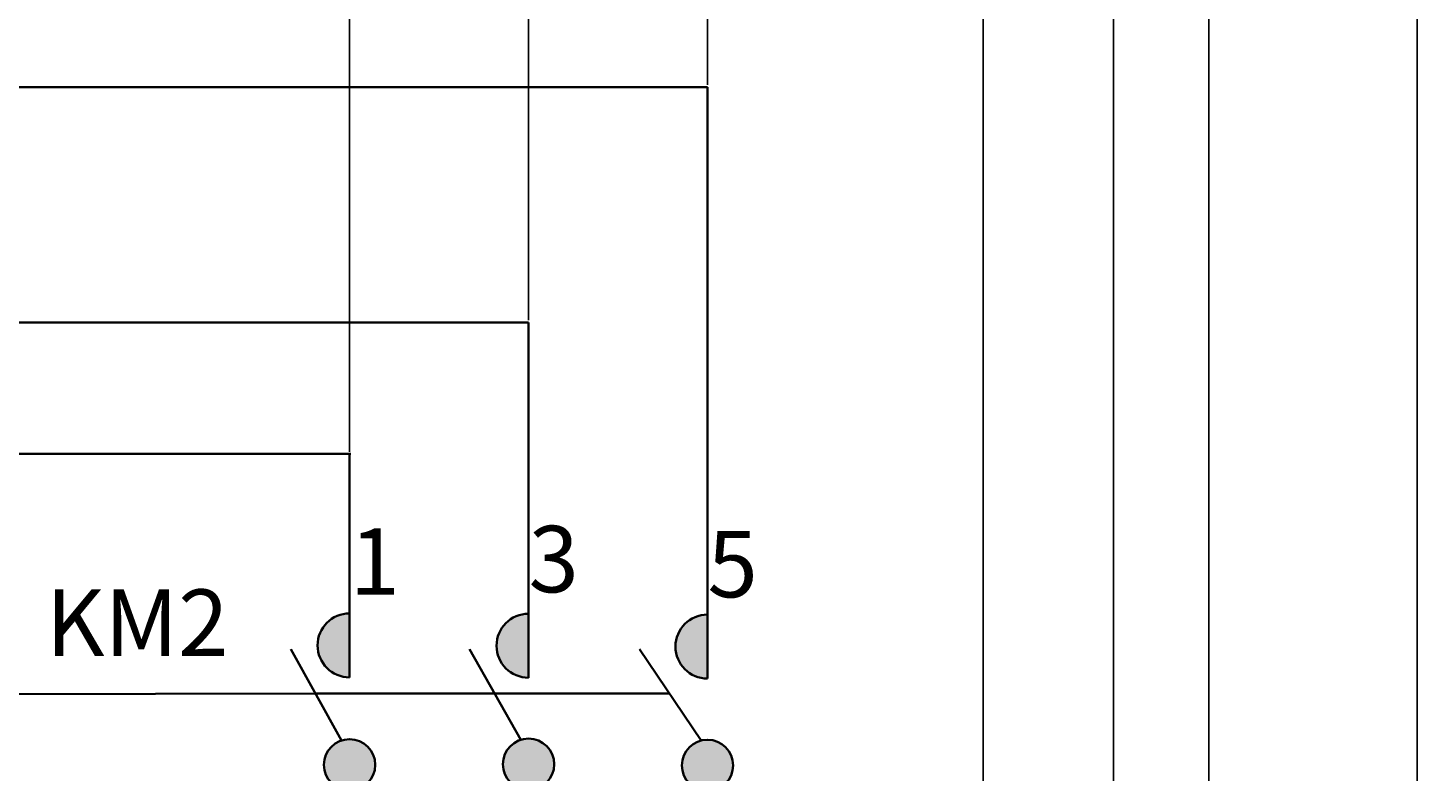
# Model space of a CAD drawing. Units: inches. Extents: x 237 to 313, y 343 to 451.
# Tile 5 of 6: x 274 to 313, y 410 to 430. Entities that reach past the tile are written whole.
import ezdxf

# ---------------------------------------------------------------- set-up
doc = ezdxf.new("R2010")
doc.units = ezdxf.units.IN
doc.header["$MEASUREMENT"] = 0
doc.layers.get('0').update_dxf_attribs({"color": 240})
for name, color, linetype, lineweight in [('A-ANNO-DIMS', 2, 'Continuous', 18), ('E-ANNO-TEXT', 7, 'Continuous', 25), ('E-DEVC', 4, 'Continuous', 35), ('E-WIRE', 7, 'Continuous', 35)]:
    doc.layers.add(name, color=color, linetype=linetype, lineweight=lineweight)
doc.styles.get("Standard").update_dxf_attribs({"font": 'arial.ttf'})
doc.dimstyles.get("Standard").update_dxf_attribs({"dimtxt": 0.18, "dimasz": 0.18, "dimexe": 0.18, "dimexo": 0.0625, "dimgap": 0.09, "dimtad": 0, "dimtih": 1, "dimtoh": 1, "dimdec": 4, "dimzin": 0, "dimdsep": 46, "dimtxsty": 'Standard', "dimcen": 0.09, "dimadec": 0, "dimazin": 0, "dimtfac": 1, "dimtdec": 4, "dimtofl": 0, "dimtmove": 0, "dimatfit": 3, "dimfxl": 1, "dimtolj": 1, "dimtzin": 0, "dimarcsym": 0})

# ---------------------------------------------------------------- blocks, each defined once
blk = doc.blocks.new('CONTACTOR-3P-NO')
h = blk.add_hatch(color=256)
h.dxf.hatch_style = 1
h.paths.add_polyline_path([(1.637, 4.965, 1), (1.637, 3.177)])
h.paths.add_polyline_path([(6.637, 4.953, 1), (6.637, 3.166)])
h.paths.add_polyline_path([(11.637, 4.931, 1), (11.637, 3.144)])
h = blk.add_hatch(color=256)
h.dxf.hatch_style = 1
h.paths.add_polyline_path([(2.354, 0.734, 1), (0.92, 0.734, 1)])
h.paths.add_polyline_path([(5.92, 0.749, 1), (7.354, 0.749, 1)])
h.paths.add_polyline_path([(10.92, 0.717, 1), (12.354, 0.717, 1)])
for p, q in [((1.414, 1.415), (0, 3.965)), ((6.423, 1.433), (4.991, 3.965)), ((11.461, 1.412), (9.739, 3.965))]:
    blk.add_line(p, q)
for centre in [(1.637, 0.734), (6.637, 0.749), (11.637, 0.717)]:
    blk.add_circle(centre, 0.717)
for centre in [(1.637, 4.071), (6.637, 4.06), (11.637, 4.037)]:
    blk.add_arc(centre, 0.894, 90, 270)
blk = doc.blocks.new('*D3')
at = {"layer": 'A-ANNO-DIMS', "color": 0, "lineweight": -2, "transparency": 16777216}
for p, q in [((242.3, 363.785), (242.3, 451.078)), ((306.656, 382.738), (306.656, 451.078)), ((242.48, 450.898), (274.084, 450.898)), ((306.476, 450.898), (274.872, 450.898))]:
    blk.add_line(p, q, dxfattribs=at)
at = {"layer": 'A-ANNO-DIMS', "color": 0, "lineweight": 35, "transparency": 16777216}
for points in [[(242.48, 450.928), (242.48, 450.868), (242.3, 450.898)], [(306.476, 450.928), (306.476, 450.868), (306.656, 450.898)]]:
    blk.add_solid(points, dxfattribs=at)
at = {"layer": 'Defpoints', "color": 0, "lineweight": 35, "transparency": 16777216}
for p in [(306.656, 450.898), (306.656, 382.675), (242.3, 363.723)]:
    blk.add_point(p, dxfattribs=at)
at = {"layer": 'A-ANNO-DIMS', "color": 0, "transparency": 16777216, "insert": (274.478, 450.898), "char_height": 0.18, "attachment_point": 5}
blk.add_mtext('\\A1;64.36', dxfattribs=at)
blk = doc.blocks.new('*D4')
at = {"layer": 'A-ANNO-DIMS', "color": 0, "lineweight": -2, "transparency": 16777216}
for p, q in [((258.115, 445.823), (312.65, 445.823)), ((312.47, 445.643), (312.47, 397.21)), ((312.47, 348.414), (312.47, 396.846)), ((289.124, 348.234), (312.65, 348.234))]:
    blk.add_line(p, q, dxfattribs=at)
at = {"layer": 'A-ANNO-DIMS', "color": 0, "lineweight": 35, "transparency": 16777216}
for points in [[(312.44, 445.643), (312.5, 445.643), (312.47, 445.823)], [(312.44, 348.414), (312.5, 348.414), (312.47, 348.234)]]:
    blk.add_solid(points, dxfattribs=at)
at = {"layer": 'Defpoints', "color": 0, "lineweight": 35, "transparency": 16777216}
for p in [(258.052, 445.823), (289.062, 348.234), (312.47, 348.234)]:
    blk.add_point(p, dxfattribs=at)
at = {"layer": 'A-ANNO-DIMS', "color": 0, "transparency": 16777216, "insert": (312.47, 397.028), "char_height": 0.18, "attachment_point": 5}
blk.add_mtext('\\A1;97.59', dxfattribs=at)
blk = doc.blocks.new('*D7')
at = {"layer": 'A-ANNO-DIMS', "color": 0, "lineweight": -2, "transparency": 16777216}
for p, q in [((257.997, 436.662), (257.997, 451.078)), ((282.648, 418.461), (282.648, 451.078)), ((258.177, 450.898), (269.926, 450.898)), ((282.468, 450.898), (270.718, 450.898))]:
    blk.add_line(p, q, dxfattribs=at)
at = {"layer": 'A-ANNO-DIMS', "color": 0, "lineweight": 35, "transparency": 16777216}
for points in [[(258.177, 450.928), (258.177, 450.868), (257.997, 450.898)], [(282.468, 450.928), (282.468, 450.868), (282.648, 450.898)]]:
    blk.add_solid(points, dxfattribs=at)
at = {"layer": 'Defpoints', "color": 0, "lineweight": 35, "transparency": 16777216}
for p in [(282.648, 450.898), (257.997, 436.599), (282.648, 418.399)]:
    blk.add_point(p, dxfattribs=at)
at = {"layer": 'A-ANNO-DIMS', "color": 0, "transparency": 16777216, "insert": (270.322, 450.898), "char_height": 0.18, "attachment_point": 5}
blk.add_mtext('\\A1;24.65', dxfattribs=at)
blk = doc.blocks.new('*D8')
at = {"layer": 'A-ANNO-DIMS', "color": 0, "lineweight": -2, "transparency": 16777216}
for p, q in [((282.648, 418.461), (282.648, 451.078)), ((287.648, 422.133), (287.648, 451.078)), ((282.828, 450.898), (284.998, 450.898)), ((287.468, 450.898), (285.297, 450.898))]:
    blk.add_line(p, q, dxfattribs=at)
at = {"layer": 'A-ANNO-DIMS', "color": 0, "lineweight": 35, "transparency": 16777216}
for points in [[(282.828, 450.928), (282.828, 450.868), (282.648, 450.898)], [(287.468, 450.928), (287.468, 450.868), (287.648, 450.898)]]:
    blk.add_solid(points, dxfattribs=at)
at = {"layer": 'Defpoints', "color": 0, "lineweight": 35, "transparency": 16777216}
for p in [(287.648, 450.898), (287.648, 422.07), (282.648, 418.399)]:
    blk.add_point(p, dxfattribs=at)
at = {"layer": 'A-ANNO-DIMS', "color": 0, "transparency": 16777216, "insert": (285.148, 450.898), "char_height": 0.18, "attachment_point": 5}
blk.add_mtext('\\A1;5', dxfattribs=at)
blk = doc.blocks.new('*D9')
at = {"layer": 'A-ANNO-DIMS', "color": 0, "lineweight": -2, "transparency": 16777216}
for p, q in [((287.648, 422.133), (287.648, 451.078)), ((292.648, 428.708), (292.648, 451.078)), ((287.828, 450.898), (289.998, 450.898)), ((292.468, 450.898), (290.297, 450.898))]:
    blk.add_line(p, q, dxfattribs=at)
at = {"layer": 'A-ANNO-DIMS', "color": 0, "lineweight": 35, "transparency": 16777216}
for points in [[(287.828, 450.928), (287.828, 450.868), (287.648, 450.898)], [(292.468, 450.928), (292.468, 450.868), (292.648, 450.898)]]:
    blk.add_solid(points, dxfattribs=at)
at = {"layer": 'Defpoints', "color": 0, "lineweight": 35, "transparency": 16777216}
for p in [(292.648, 450.898), (292.648, 428.646), (287.648, 422.07)]:
    blk.add_point(p, dxfattribs=at)
at = {"layer": 'A-ANNO-DIMS', "color": 0, "transparency": 16777216, "insert": (290.148, 450.898), "char_height": 0.18, "attachment_point": 5}
blk.add_mtext('\\A1;5', dxfattribs=at)
blk = doc.blocks.new('*D10')
at = {"layer": 'A-ANNO-DIMS', "color": 0, "lineweight": -2, "transparency": 16777216}
for p, q in [((300.353, 382.738), (300.353, 451.078)), ((303.989, 382.738), (303.989, 451.078)), ((300.533, 450.898), (301.848, 450.898)), ((303.809, 450.898), (302.495, 450.898))]:
    blk.add_line(p, q, dxfattribs=at)
at = {"layer": 'A-ANNO-DIMS', "color": 0, "lineweight": 35, "transparency": 16777216}
for points in [[(300.533, 450.928), (300.533, 450.868), (300.353, 450.898)], [(303.809, 450.928), (303.809, 450.868), (303.989, 450.898)]]:
    blk.add_solid(points, dxfattribs=at)
at = {"layer": 'Defpoints', "color": 0, "lineweight": 35, "transparency": 16777216}
for p in [(303.989, 450.898), (300.353, 382.675), (303.989, 382.675)]:
    blk.add_point(p, dxfattribs=at)
at = {"layer": 'A-ANNO-DIMS', "color": 0, "transparency": 16777216, "insert": (302.171, 450.898), "char_height": 0.18, "attachment_point": 5}
blk.add_mtext('\\A1;3.64', dxfattribs=at)
blk = doc.blocks.new('*D11')
at = {"layer": 'A-ANNO-DIMS', "color": 0, "lineweight": -2, "transparency": 16777216}
for p, q in [((303.989, 382.738), (303.989, 451.078)), ((306.656, 382.738), (306.656, 451.078)), ((304.169, 450.898), (304.928, 450.898)), ((306.476, 450.898), (305.718, 450.898))]:
    blk.add_line(p, q, dxfattribs=at)
at = {"layer": 'A-ANNO-DIMS', "color": 0, "lineweight": 35, "transparency": 16777216}
for points in [[(304.169, 450.928), (304.169, 450.868), (303.989, 450.898)], [(306.476, 450.928), (306.476, 450.868), (306.656, 450.898)]]:
    blk.add_solid(points, dxfattribs=at)
at = {"layer": 'Defpoints', "color": 0, "lineweight": 35, "transparency": 16777216}
for p in [(306.656, 450.898), (303.989, 382.675), (306.656, 382.675)]:
    blk.add_point(p, dxfattribs=at)
at = {"layer": 'A-ANNO-DIMS', "color": 0, "transparency": 16777216, "insert": (305.323, 450.898), "char_height": 0.18, "attachment_point": 5}
blk.add_mtext('\\A1;2.667', dxfattribs=at)

msp = doc.modelspace()

# ---------------------------------------------------------------- linework, layer by layer
at = {"layer": 'E-DEVC'}
for p, q in [((270.552, 411.6855), (281.6957, 411.7099)), ((281.6957, 411.7099), (291.5864, 411.705))]:
    msp.add_line(p, q, dxfattribs=at)
at = {"layer": 'E-WIRE'}
for p, q in [((259.5057, 428.6459), (292.6477, 428.6459)), ((292.6477, 428.6459), (292.6477, 412.1237)), ((254.5187, 422.0704), (287.6477, 422.0704)), ((287.6477, 422.0704), (287.6477, 412.1461)), ((249.4968, 418.3988), (282.6795, 418.3988)), ((282.6477, 418.3988), (282.6477, 412.1574))]:
    msp.add_line(p, q, dxfattribs=at)

# ---------------------------------------------------------------- block references
at = {"layer": 'E-DEVC'}
msp.add_blockref('CONTACTOR-3P-NO', (281.0109, 408.98), dxfattribs=at)

# ---------------------------------------------------------------- texts
at = {"layer": 'E-ANNO-TEXT'}
for s, height, p in [('1', 1.8564, (282.6477, 414.4631)), ('3', 1.8564, (287.6477, 414.533)), ('5', 1.8564, (292.6477, 414.3932)), ('KM2', 1.85645, (274.1673, 412.7559))]:
    msp.add_text(s, height=height, dxfattribs=at).set_placement(p)

# ---------------------------------------------------------------- dimensions: what is measured, and where the dimension line sits
at = {"layer": 'A-ANNO-DIMS'}
for base, p1, p2, override, picture, middle in [((306.6564, 450.8976), (242.3002, 363.7227), (306.6564, 382.675), {"dimdec": 2, "dimlfac": 1, "dimrnd": 0, "dimzin": 0, "dimdsep": 46, "dimlunit": 2}, '*D3', (274.4783, 450.8976)), ((282.6477, 450.8976), (257.9968, 436.5992), (282.6477, 418.3988), {"dimdec": 2, "dimlfac": 1, "dimrnd": 0, "dimzin": 0, "dimdsep": 46, "dimlunit": 2}, '*D7', (270.3223, 450.8976)), ((287.6477, 450.8976), (282.6477, 418.3988), (287.6477, 422.0704), {"dimdec": 0, "dimlfac": 1, "dimrnd": 0, "dimzin": 0, "dimdsep": 46, "dimlunit": 2}, '*D8', (285.1477, 450.8976)), ((292.6477, 450.8976), (287.6477, 422.0704), (292.6477, 428.6459), {"dimdec": 0, "dimlfac": 1, "dimrnd": 0, "dimzin": 0, "dimdsep": 46, "dimlunit": 2}, '*D9', (290.1477, 450.8976)), ((303.9895, 450.8976), (300.3529, 382.675), (303.9895, 382.675), {"dimdec": 2, "dimlfac": 1, "dimrnd": 0, "dimzin": 0, "dimdsep": 46, "dimlunit": 2}, '*D10', (302.1712, 450.8976)), ((306.6564, 450.8976), (303.9895, 382.675), (306.6564, 382.675), {"dimdec": 3, "dimlfac": 1, "dimrnd": 0, "dimzin": 0, "dimdsep": 46, "dimlunit": 2}, '*D11', (305.3229, 450.8976))]:
    dim = msp.add_linear_dim(base=base, p1=p1, p2=p2, dimstyle='Standard', override=override, dxfattribs=at)
    dim.commit()
    dim.dimension.update_dxf_attribs({"geometry": picture, "text_midpoint": middle})
dim = msp.add_linear_dim(base=(312.4701, 348.2337), p1=(258.0525, 445.8226), p2=(289.0615, 348.2337), angle=90, dimstyle='Standard', override={"dimdec": 2, "dimlfac": 1, "dimrnd": 0, "dimzin": 0, "dimdsep": 46, "dimlunit": 2}, dxfattribs=at)
dim.commit()
dim.dimension.update_dxf_attribs({"geometry": '*D4', "text_midpoint": (312.4701, 397.0282)})

doc.saveas('drawing.dxf')
